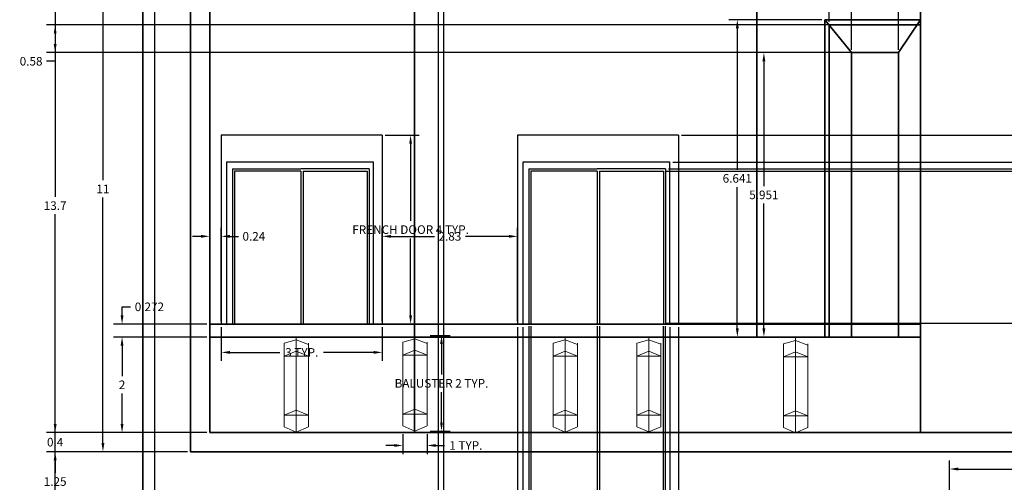
# Model space of a CAD drawing. Units: millimetres. Extents: x 2473 to 2512.3, y 2191.3 to 2230.4.
# Tile 3 of 8: x 2473 to 2493.7, y 2206.4 to 2216.1. Entities that reach past the tile are written whole.
import ezdxf

# ---------------------------------------------------------------- set-up
doc = ezdxf.new("R2010")
doc.units = ezdxf.units.MM
for name, color, linetype, lineweight in [('A-ANNO-DIMS', 2, 'Continuous', 18), ('A-ELEV', 7, 'Continuous', 35), ('A-FLOR-HRAL', 8, 'Continuous', 18), ('A-GLAZ', 3, 'Continuous', 25)]:
    doc.layers.add(name, color=color, linetype=linetype, lineweight=lineweight)
doc.styles.get("Standard").update_dxf_attribs({"font": 'arial.ttf'})
doc.dimstyles.get("Standard").update_dxf_attribs({"dimtxt": 0.18, "dimasz": 0.18, "dimexe": 0.18, "dimexo": 0.0625, "dimgap": 0.09, "dimtad": 0, "dimtih": 1, "dimtoh": 1, "dimdec": 4, "dimzin": 0, "dimdsep": 46, "dimtxsty": 'Standard', "dimcen": 0.09, "dimadec": 0, "dimazin": 0, "dimtfac": 1, "dimtdec": 4, "dimtofl": 0, "dimtmove": 0, "dimatfit": 3, "dimfxl": 1, "dimtolj": 1, "dimtzin": 0, "dimarcsym": 0})

# ---------------------------------------------------------------- blocks, each defined once
blk = doc.blocks.new('BALUSTER')
for p, q in [((0, 1.86), (0.25, 1.93)), ((0, 1.86), (0, 0.108)), ((0.25, 2), (0.25, 0)), ((0.25, 1.93), (0.507, 1.835)), ((0.507, 0.108), (0.507, 1.86)), ((0, 1.589), (0.25, 1.693)), ((0.25, 1.693), (0.507, 1.589)), ((0, 1.589), (0.25, 1.589)), ((0.25, 1.589), (0.507, 1.589)), ((0, 0.354), (0.25, 0.459)), ((0.25, 0.459), (0.507, 0.354)), ((0, 0.354), (0.25, 0.354)), ((0.25, 0.354), (0.507, 0.354)), ((0.25, 0), (0, 0.108)), ((0.25, 0), (0.507, 0.108))]:
    blk.add_line(p, q)
blk = doc.blocks.new('WIN-FRENCH-DOOR')
for p, q in [((0, 3.953), (0, 0)), ((3.371, 3.953), (0, 3.953)), ((3.371, 3.953), (3.371, 0)), ((3.186, 3.385), (0.113, 3.385)), ((0.113, 3.385), (0.113, 0)), ((3.186, 0), (3.186, 3.385)), ((0.234, 3.25), (0.234, 0.02)), ((0.234, 3.25), (1.664, 3.25)), ((1.664, 3.2), (0.275, 3.2)), ((0.275, 3.2), (0.275, 0.02)), ((3.094, 3.25), (1.664, 3.25)), ((1.664, 3.2), (1.664, 0.02)), ((1.664, 3.2), (1.664, 0.02)), ((1.718, 3.2), (3.052, 3.2)), ((1.718, 3.2), (1.718, 0.016)), ((3.052, 3.2), (3.052, 0.02)), ((3.094, 3.25), (3.094, 0.02))]:
    blk.add_line(p, q)
blk = doc.blocks.new('*D3')
at = {"layer": 'A-ANNO-DIMS', "color": 0, "lineweight": -2, "transparency": 16777216}
for p, q in [((2481.638, 2209.486), (2482.056, 2209.486)), ((2481.876, 2209.306), (2481.876, 2208.669)), ((2481.876, 2207.666), (2481.876, 2208.303)), ((2481.638, 2207.486), (2482.056, 2207.486))]:
    blk.add_line(p, q, dxfattribs=at)
at = {"layer": 'A-ANNO-DIMS', "color": 0, "transparency": 16777216}
for points in [[(2481.846, 2209.306), (2481.906, 2209.306), (2481.876, 2209.486)], [(2481.846, 2207.666), (2481.906, 2207.666), (2481.876, 2207.486)]]:
    blk.add_solid(points, dxfattribs=at)
at = {"layer": 'Defpoints', "color": 0, "transparency": 16777216}
for p in [(2481.576, 2209.486), (2481.876, 2209.486), (2481.576, 2207.486)]:
    blk.add_point(p, dxfattribs=at)
at = {"layer": 'A-ANNO-DIMS', "color": 0, "transparency": 16777216, "insert": (2481.876, 2208.486), "char_height": 0.18, "attachment_point": 5}
blk.add_mtext('\\A1;BALUSTER 2 TYP.', dxfattribs=at)
blk = doc.blocks.new('*D4')
at = {"layer": 'A-ANNO-DIMS', "color": 0, "lineweight": -2, "transparency": 16777216}
for p, q in [((2481.069, 2207.423), (2481.069, 2207.006)), ((2481.576, 2207.423), (2481.576, 2207.006)), ((2480.889, 2207.186), (2480.709, 2207.186)), ((2481.756, 2207.186), (2481.936, 2207.186))]:
    blk.add_line(p, q, dxfattribs=at)
at = {"layer": 'A-ANNO-DIMS', "color": 0, "transparency": 16777216}
for points in [[(2480.889, 2207.216), (2480.889, 2207.156), (2481.069, 2207.186)], [(2481.756, 2207.216), (2481.756, 2207.156), (2481.576, 2207.186)]]:
    blk.add_solid(points, dxfattribs=at)
at = {"layer": 'Defpoints', "color": 0, "transparency": 16777216}
for p in [(2481.069, 2207.486), (2481.576, 2207.486), (2481.576, 2207.186)]:
    blk.add_point(p, dxfattribs=at)
at = {"layer": 'A-ANNO-DIMS', "color": 0, "transparency": 16777216, "insert": (2482.386, 2207.186), "char_height": 0.18, "attachment_point": 5}
blk.add_mtext('\\A1;1 TYP.', dxfattribs=at)
blk = doc.blocks.new('*D5')
at = {"layer": 'A-ANNO-DIMS', "color": 0, "lineweight": -2, "transparency": 16777216}
for p, q in [((2480.698, 2213.68), (2481.409, 2213.68)), ((2481.229, 2213.5), (2481.229, 2211.886)), ((2481.229, 2209.907), (2481.229, 2211.52)), ((2480.698, 2209.727), (2481.409, 2209.727))]:
    blk.add_line(p, q, dxfattribs=at)
at = {"layer": 'A-ANNO-DIMS', "color": 0, "transparency": 16777216}
for points in [[(2481.199, 2213.5), (2481.259, 2213.5), (2481.229, 2213.68)], [(2481.199, 2209.907), (2481.259, 2209.907), (2481.229, 2209.727)]]:
    blk.add_solid(points, dxfattribs=at)
at = {"layer": 'Defpoints', "color": 0, "transparency": 16777216}
for p in [(2480.636, 2213.68), (2481.229, 2213.68), (2480.636, 2209.727)]:
    blk.add_point(p, dxfattribs=at)
at = {"layer": 'A-ANNO-DIMS', "color": 0, "transparency": 16777216, "insert": (2481.229, 2211.703), "char_height": 0.18, "attachment_point": 5}
blk.add_mtext('\\A1;FRENCH DOOR 4 TYP.', dxfattribs=at)
blk = doc.blocks.new('*D6')
at = {"layer": 'A-ANNO-DIMS', "color": 0, "lineweight": -2, "transparency": 16777216}
for p, q in [((2477.265, 2209.664), (2477.265, 2208.954)), ((2480.636, 2209.664), (2480.636, 2208.954)), ((2477.445, 2209.134), (2478.492, 2209.134)), ((2480.456, 2209.134), (2479.408, 2209.134))]:
    blk.add_line(p, q, dxfattribs=at)
at = {"layer": 'A-ANNO-DIMS', "color": 0, "transparency": 16777216}
for points in [[(2477.445, 2209.164), (2477.445, 2209.104), (2477.265, 2209.134)], [(2480.456, 2209.164), (2480.456, 2209.104), (2480.636, 2209.134)]]:
    blk.add_solid(points, dxfattribs=at)
at = {"layer": 'Defpoints', "color": 0, "transparency": 16777216}
for p in [(2477.265, 2209.727), (2480.636, 2209.727), (2480.636, 2209.134)]:
    blk.add_point(p, dxfattribs=at)
at = {"layer": 'A-ANNO-DIMS', "color": 0, "transparency": 16777216, "insert": (2478.95, 2209.134), "char_height": 0.18, "attachment_point": 5}
blk.add_mtext('\\A1;3 TYP.', dxfattribs=at)
blk = doc.blocks.new('*D12')
at = {"layer": 'A-ANNO-DIMS', "color": 0, "lineweight": -2, "transparency": 16777216}
for p, q in [((2475.56, 2219.055), (2473.608, 2219.055)), ((2473.788, 2218.875), (2473.788, 2212.387)), ((2473.788, 2205.535), (2473.788, 2212.023)), ((2475.56, 2205.355), (2473.608, 2205.355))]:
    blk.add_line(p, q, dxfattribs=at)
at = {"layer": 'A-ANNO-DIMS', "color": 0, "transparency": 16777216}
for points in [[(2473.758, 2218.875), (2473.818, 2218.875), (2473.788, 2219.055)], [(2473.758, 2205.535), (2473.818, 2205.535), (2473.788, 2205.355)]]:
    blk.add_solid(points, dxfattribs=at)
at = {"layer": 'Defpoints', "color": 0, "transparency": 16777216}
for p in [(2473.788, 2219.055), (2475.623, 2219.055), (2475.623, 2205.355)]:
    blk.add_point(p, dxfattribs=at)
at = {"layer": 'A-ANNO-DIMS', "color": 0, "transparency": 16777216, "insert": (2473.788, 2212.205), "char_height": 0.18, "attachment_point": 5}
blk.add_mtext('\\A1;13.7', dxfattribs=at)
blk = doc.blocks.new('*D19')
at = {"layer": 'A-ANNO-DIMS', "color": 0, "lineweight": -2, "transparency": 16777216}
for p, q in [((2476.56, 2218.055), (2474.608, 2218.055)), ((2474.788, 2217.875), (2474.788, 2212.735)), ((2474.788, 2207.235), (2474.788, 2212.375)), ((2476.56, 2207.055), (2474.608, 2207.055))]:
    blk.add_line(p, q, dxfattribs=at)
at = {"layer": 'A-ANNO-DIMS', "color": 0, "transparency": 16777216}
for points in [[(2474.758, 2217.875), (2474.818, 2217.875), (2474.788, 2218.055)], [(2474.758, 2207.235), (2474.818, 2207.235), (2474.788, 2207.055)]]:
    blk.add_solid(points, dxfattribs=at)
at = {"layer": 'Defpoints', "color": 0, "transparency": 16777216}
for p in [(2474.788, 2218.055), (2476.623, 2218.055), (2476.623, 2207.055)]:
    blk.add_point(p, dxfattribs=at)
at = {"layer": 'A-ANNO-DIMS', "color": 0, "transparency": 16777216, "insert": (2474.788, 2212.555), "char_height": 0.18, "attachment_point": 5}
blk.add_mtext('\\A1;11', dxfattribs=at)
blk = doc.blocks.new('*D38')
at = {"layer": 'A-ANNO-DIMS', "color": 0, "lineweight": -2, "transparency": 16777216}
for p, q in [((2476.56, 2207.055), (2473.608, 2207.055)), ((2473.788, 2206.875), (2473.788, 2206.613)), ((2473.788, 2205.988), (2473.788, 2206.249)), ((2475.56, 2205.808), (2473.608, 2205.808))]:
    blk.add_line(p, q, dxfattribs=at)
at = {"layer": 'A-ANNO-DIMS', "color": 0, "transparency": 16777216}
for points in [[(2473.758, 2206.875), (2473.818, 2206.875), (2473.788, 2207.055)], [(2473.758, 2205.988), (2473.818, 2205.988), (2473.788, 2205.808)]]:
    blk.add_solid(points, dxfattribs=at)
at = {"layer": 'Defpoints', "color": 0, "transparency": 16777216}
for p in [(2473.788, 2207.055), (2476.623, 2207.055), (2475.623, 2205.808)]:
    blk.add_point(p, dxfattribs=at)
at = {"layer": 'A-ANNO-DIMS', "color": 0, "transparency": 16777216, "insert": (2473.788, 2206.431), "char_height": 0.18, "attachment_point": 5}
blk.add_mtext('\\A1;1.25', dxfattribs=at)
blk = doc.blocks.new('*D44')
at = {"layer": 'A-ANNO-DIMS', "color": 0, "lineweight": -2, "transparency": 16777216}
for p, q in [((2492.513, 2204.92), (2492.513, 2206.873)), ((2499.711, 2204.92), (2499.711, 2206.873)), ((2492.693, 2206.693), (2495.719, 2206.693)), ((2499.531, 2206.693), (2496.505, 2206.693))]:
    blk.add_line(p, q, dxfattribs=at)
at = {"layer": 'A-ANNO-DIMS', "color": 0, "transparency": 16777216}
for points in [[(2492.693, 2206.723), (2492.693, 2206.663), (2492.513, 2206.693)], [(2499.531, 2206.723), (2499.531, 2206.663), (2499.711, 2206.693)]]:
    blk.add_solid(points, dxfattribs=at)
at = {"layer": 'Defpoints', "color": 0, "transparency": 16777216}
for p in [(2499.711, 2206.693), (2492.513, 2204.858), (2499.711, 2204.858)]:
    blk.add_point(p, dxfattribs=at)
at = {"layer": 'A-ANNO-DIMS', "color": 0, "transparency": 16777216, "insert": (2496.112, 2206.693), "char_height": 0.18, "attachment_point": 5}
blk.add_mtext('\\A1;7.197', dxfattribs=at)
blk = doc.blocks.new('*D45')
at = {"layer": 'A-ANNO-DIMS', "color": 0, "lineweight": -2, "transparency": 16777216}
for p, q in [((2473.787904, 2207.634888), (2473.787904, 2207.814888)), ((2476.960404, 2207.454888), (2473.607904, 2207.454888)), ((2476.560404, 2207.054888), (2473.607904, 2207.054888)), ((2473.787904, 2206.874888), (2473.787904, 2206.694888))]:
    blk.add_line(p, q, dxfattribs=at)
at = {"layer": 'A-ANNO-DIMS', "color": 0, "transparency": 16777216}
for points in [[(2473.757904, 2207.634888), (2473.817904, 2207.634888), (2473.787904, 2207.454888)], [(2473.757904, 2206.874888), (2473.817904, 2206.874888), (2473.787904, 2207.054888)]]:
    blk.add_solid(points, dxfattribs=at)
at = {"layer": 'Defpoints', "color": 0, "transparency": 16777216}
for p in [(2473.787904, 2207.454888), (2477.022904, 2207.454888), (2476.622904, 2207.054888)]:
    blk.add_point(p, dxfattribs=at)
at = {"layer": 'A-ANNO-DIMS', "color": 0, "transparency": 16777216, "insert": (2473.787904, 2207.254888), "char_height": 0.18, "attachment_point": 5}
blk.add_mtext('\\A1;0.4', dxfattribs=at)
blk = doc.blocks.new('*D52')
at = {"layer": 'A-ANNO-DIMS', "color": 0, "lineweight": -2, "transparency": 16777216}
for p, q in [((2477.023, 2209.789), (2477.023, 2211.742)), ((2477.265, 2209.789), (2477.265, 2211.742)), ((2476.843, 2211.562), (2476.663, 2211.562)), ((2477.445, 2211.562), (2477.625, 2211.562))]:
    blk.add_line(p, q, dxfattribs=at)
at = {"layer": 'A-ANNO-DIMS', "color": 0, "transparency": 16777216}
for points in [[(2476.843, 2211.592), (2476.843, 2211.532), (2477.023, 2211.562)], [(2477.445, 2211.592), (2477.445, 2211.532), (2477.265, 2211.562)]]:
    blk.add_solid(points, dxfattribs=at)
at = {"layer": 'Defpoints', "color": 0, "transparency": 16777216}
for p in [(2477.265, 2211.562), (2477.023, 2209.727), (2477.265, 2209.727)]:
    blk.add_point(p, dxfattribs=at)
at = {"layer": 'A-ANNO-DIMS', "color": 0, "transparency": 16777216, "insert": (2477.948, 2211.562), "char_height": 0.18, "attachment_point": 5}
blk.add_mtext('\\A1;0.24', dxfattribs=at)
blk = doc.blocks.new('*D53')
at = {"layer": 'A-ANNO-DIMS', "color": 0, "lineweight": -2, "transparency": 16777216}
for p, q in [((2480.636, 2209.789), (2480.636, 2211.742)), ((2483.468, 2209.789), (2483.468, 2211.742)), ((2480.816, 2211.562), (2481.727, 2211.562)), ((2483.288, 2211.562), (2482.377, 2211.562))]:
    blk.add_line(p, q, dxfattribs=at)
at = {"layer": 'A-ANNO-DIMS', "color": 0, "transparency": 16777216}
for points in [[(2480.816, 2211.592), (2480.816, 2211.532), (2480.636, 2211.562)], [(2483.288, 2211.592), (2483.288, 2211.532), (2483.468, 2211.562)]]:
    blk.add_solid(points, dxfattribs=at)
at = {"layer": 'Defpoints', "color": 0, "transparency": 16777216}
for p in [(2483.468, 2211.562), (2480.636, 2209.727), (2483.468, 2209.727)]:
    blk.add_point(p, dxfattribs=at)
at = {"layer": 'A-ANNO-DIMS', "color": 0, "transparency": 16777216, "insert": (2482.052, 2211.562), "char_height": 0.18, "attachment_point": 5}
blk.add_mtext('\\A1;2.83', dxfattribs=at)
blk = doc.blocks.new('*D54')
at = {"layer": 'A-ANNO-DIMS', "color": 0, "lineweight": -2, "transparency": 16777216}
for p, q in [((2476.96, 2209.455), (2475.008, 2209.455)), ((2475.188, 2209.275), (2475.188, 2208.635)), ((2475.188, 2207.635), (2475.188, 2208.275)), ((2476.96, 2207.455), (2475.008, 2207.455))]:
    blk.add_line(p, q, dxfattribs=at)
at = {"layer": 'A-ANNO-DIMS', "color": 0, "transparency": 16777216}
for points in [[(2475.158, 2209.275), (2475.218, 2209.275), (2475.188, 2209.455)], [(2475.158, 2207.635), (2475.218, 2207.635), (2475.188, 2207.455)]]:
    blk.add_solid(points, dxfattribs=at)
at = {"layer": 'Defpoints', "color": 0, "transparency": 16777216}
for p in [(2475.188, 2209.455), (2477.023, 2209.455), (2477.023, 2207.455)]:
    blk.add_point(p, dxfattribs=at)
at = {"layer": 'A-ANNO-DIMS', "color": 0, "transparency": 16777216, "insert": (2475.188, 2208.455), "char_height": 0.18, "attachment_point": 5}
blk.add_mtext('\\A1;2', dxfattribs=at)
blk = doc.blocks.new('*D55')
at = {"layer": 'A-ANNO-DIMS', "color": 0, "lineweight": -2, "transparency": 16777216}
for p, q in [((2475.188, 2209.907), (2475.188, 2210.087)), ((2475.188, 2210.087), (2475.368, 2210.087)), ((2476.96, 2209.727), (2475.008, 2209.727)), ((2476.96, 2209.455), (2475.008, 2209.455)), ((2475.188, 2209.275), (2475.188, 2209.095))]:
    blk.add_line(p, q, dxfattribs=at)
at = {"layer": 'A-ANNO-DIMS', "color": 0, "transparency": 16777216}
for points in [[(2475.158, 2209.907), (2475.218, 2209.907), (2475.188, 2209.727)], [(2475.158, 2209.275), (2475.218, 2209.275), (2475.188, 2209.455)]]:
    blk.add_solid(points, dxfattribs=at)
at = {"layer": 'Defpoints', "color": 0, "transparency": 16777216}
for p in [(2475.188, 2209.727), (2477.023, 2209.727), (2477.023, 2209.455)]:
    blk.add_point(p, dxfattribs=at)
at = {"layer": 'A-ANNO-DIMS', "color": 0, "transparency": 16777216, "insert": (2475.761, 2210.087), "char_height": 0.18, "attachment_point": 5}
blk.add_mtext('\\A1;0.272', dxfattribs=at)
blk = doc.blocks.new('*D58')
at = {"layer": 'A-ANNO-DIMS', "color": 0, "lineweight": -2, "transparency": 16777216}
for p, q in [((2490.46, 2215.468), (2490.46, 2217.421)), ((2491.441, 2215.468), (2491.441, 2217.421)), ((2490.28, 2217.241), (2490.1, 2217.241)), ((2491.621, 2217.241), (2491.801, 2217.241))]:
    blk.add_line(p, q, dxfattribs=at)
at = {"layer": 'A-ANNO-DIMS', "color": 0, "transparency": 16777216}
for points in [[(2490.28, 2217.271), (2490.28, 2217.211), (2490.46, 2217.241)], [(2491.621, 2217.271), (2491.621, 2217.211), (2491.441, 2217.241)]]:
    blk.add_solid(points, dxfattribs=at)
at = {"layer": 'Defpoints', "color": 0, "transparency": 16777216}
for p in [(2491.441, 2217.241), (2490.46, 2215.406), (2491.441, 2215.406)]:
    blk.add_point(p, dxfattribs=at)
at = {"layer": 'A-ANNO-DIMS', "color": 0, "transparency": 16777216, "insert": (2490.95, 2217.241), "char_height": 0.18, "attachment_point": 5}
blk.add_mtext('\\A1;0.981', dxfattribs=at)
blk = doc.blocks.new('*D59')
at = {"layer": 'A-ANNO-DIMS', "color": 0, "lineweight": -2, "transparency": 16777216}
for p, q in [((2489.841, 2216.096), (2487.889, 2216.096)), ((2488.069, 2215.916), (2488.069, 2212.957)), ((2488.069, 2209.635), (2488.069, 2212.593)), ((2489.841, 2209.455), (2487.889, 2209.455))]:
    blk.add_line(p, q, dxfattribs=at)
at = {"layer": 'A-ANNO-DIMS', "color": 0, "transparency": 16777216}
for points in [[(2488.039, 2215.916), (2488.099, 2215.916), (2488.069, 2216.096)], [(2488.039, 2209.635), (2488.099, 2209.635), (2488.069, 2209.455)]]:
    blk.add_solid(points, dxfattribs=at)
at = {"layer": 'Defpoints', "color": 0, "transparency": 16777216}
for p in [(2488.069, 2216.096), (2489.904, 2216.096), (2489.904, 2209.455)]:
    blk.add_point(p, dxfattribs=at)
at = {"layer": 'A-ANNO-DIMS', "color": 0, "transparency": 16777216, "insert": (2488.069, 2212.775), "char_height": 0.18, "attachment_point": 5}
blk.add_mtext('\\A1;6.641', dxfattribs=at)
blk = doc.blocks.new('*D60')
at = {"layer": 'A-ANNO-DIMS', "color": 0, "lineweight": -2, "transparency": 16777216}
for p, q in [((2490.397, 2215.406), (2488.445, 2215.406)), ((2488.625, 2215.226), (2488.625, 2212.612)), ((2488.625, 2209.635), (2488.625, 2212.249)), ((2490.397, 2209.455), (2488.445, 2209.455))]:
    blk.add_line(p, q, dxfattribs=at)
at = {"layer": 'A-ANNO-DIMS', "color": 0, "transparency": 16777216}
for points in [[(2488.595, 2215.226), (2488.655, 2215.226), (2488.625, 2215.406)], [(2488.595, 2209.635), (2488.655, 2209.635), (2488.625, 2209.455)]]:
    blk.add_solid(points, dxfattribs=at)
at = {"layer": 'Defpoints', "color": 0, "transparency": 16777216}
for p in [(2488.625, 2215.406), (2490.46, 2215.406), (2490.46, 2209.455)]:
    blk.add_point(p, dxfattribs=at)
at = {"layer": 'A-ANNO-DIMS', "color": 0, "transparency": 16777216, "insert": (2488.625, 2212.43), "char_height": 0.18, "attachment_point": 5}
blk.add_mtext('\\A1;5.951', dxfattribs=at)
blk = doc.blocks.new('*D99')
at = {"layer": 'A-ANNO-DIMS', "color": 0, "lineweight": -2, "transparency": 16777216}
for p, q in [((2491.841, 2215.987), (2473.608, 2215.987)), ((2473.788, 2215.807), (2473.788, 2215.586)), ((2491.378, 2215.406), (2473.608, 2215.406)), ((2473.788, 2215.406), (2473.788, 2215.226)), ((2473.788, 2215.226), (2473.608, 2215.226))]:
    blk.add_line(p, q, dxfattribs=at)
at = {"layer": 'A-ANNO-DIMS', "color": 0, "transparency": 16777216}
for points in [[(2473.758, 2215.807), (2473.818, 2215.807), (2473.788, 2215.987)], [(2473.758, 2215.586), (2473.818, 2215.586), (2473.788, 2215.406)]]:
    blk.add_solid(points, dxfattribs=at)
at = {"layer": 'Defpoints', "color": 0, "transparency": 16777216}
for p in [(2491.904, 2215.987), (2473.788, 2215.406), (2491.441, 2215.406)]:
    blk.add_point(p, dxfattribs=at)
at = {"layer": 'A-ANNO-DIMS', "color": 0, "transparency": 16777216, "insert": (2473.284, 2215.226), "char_height": 0.18, "attachment_point": 5}
blk.add_mtext('\\A1;0.58', dxfattribs=at)
blk = doc.blocks.new('*D100')
at = {"layer": 'A-ANNO-DIMS', "color": 0, "lineweight": -2, "transparency": 16777216}
for p, q in [((2489.991, 2216.05), (2489.991, 2230.37)), ((2490.46, 2215.468), (2490.46, 2230.37)), ((2489.811, 2230.19), (2489.631, 2230.19)), ((2490.64, 2230.19), (2490.82, 2230.19))]:
    blk.add_line(p, q, dxfattribs=at)
at = {"layer": 'A-ANNO-DIMS', "color": 0, "transparency": 16777216}
for points in [[(2489.811, 2230.22), (2489.811, 2230.16), (2489.991, 2230.19)], [(2490.64, 2230.22), (2490.64, 2230.16), (2490.46, 2230.19)]]:
    blk.add_solid(points, dxfattribs=at)
at = {"layer": 'Defpoints', "color": 0, "transparency": 16777216}
for p in [(2490.46, 2230.19), (2489.991, 2215.987), (2490.46, 2215.406)]:
    blk.add_point(p, dxfattribs=at)
at = {"layer": 'A-ANNO-DIMS', "color": 0, "transparency": 16777216, "insert": (2491.143, 2230.19), "char_height": 0.18, "attachment_point": 5}
blk.add_mtext('\\A1;0.47', dxfattribs=at)
blk = doc.blocks.new('*D101')
at = {"layer": 'A-ANNO-DIMS', "color": 0, "lineweight": -2, "transparency": 16777216}
for p, q in [((2491.441, 2215.468), (2491.441, 2230.37)), ((2491.904, 2216.05), (2491.904, 2230.37)), ((2491.261, 2230.19), (2491.081, 2230.19)), ((2492.084, 2230.19), (2492.264, 2230.19))]:
    blk.add_line(p, q, dxfattribs=at)
at = {"layer": 'A-ANNO-DIMS', "color": 0, "transparency": 16777216}
for points in [[(2491.261, 2230.22), (2491.261, 2230.16), (2491.441, 2230.19)], [(2492.084, 2230.22), (2492.084, 2230.16), (2491.904, 2230.19)]]:
    blk.add_solid(points, dxfattribs=at)
at = {"layer": 'Defpoints', "color": 0, "transparency": 16777216}
for p in [(2491.904, 2230.19), (2491.904, 2215.987), (2491.441, 2215.406)]:
    blk.add_point(p, dxfattribs=at)
at = {"layer": 'A-ANNO-DIMS', "color": 0, "transparency": 16777216, "insert": (2492.587, 2230.19), "char_height": 0.18, "attachment_point": 5}
blk.add_mtext('\\A1;0.46', dxfattribs=at)
blk = doc.blocks.new('*D102')
at = {"layer": 'A-ANNO-DIMS', "color": 0, "lineweight": -2, "transparency": 16777216}
for p, q in [((2483.468, 2209.664), (2483.468, 2191.34)), ((2483.581, 2209.664), (2483.581, 2191.34)), ((2483.288, 2191.52), (2483.108, 2191.52)), ((2483.761, 2191.52), (2483.941, 2191.52))]:
    blk.add_line(p, q, dxfattribs=at)
at = {"layer": 'A-ANNO-DIMS', "color": 0, "transparency": 16777216}
for points in [[(2483.288, 2191.55), (2483.288, 2191.49), (2483.468, 2191.52)], [(2483.761, 2191.55), (2483.761, 2191.49), (2483.581, 2191.52)]]:
    blk.add_solid(points, dxfattribs=at)
at = {"layer": 'Defpoints', "color": 0, "transparency": 16777216}
for p in [(2483.468, 2209.727), (2483.581, 2209.727), (2483.581, 2191.52)]:
    blk.add_point(p, dxfattribs=at)
at = {"layer": 'A-ANNO-DIMS', "color": 0, "transparency": 16777216, "insert": (2484.248, 2191.52), "char_height": 0.18, "attachment_point": 5}
blk.add_mtext('\\A1;0.11', dxfattribs=at)
blk = doc.blocks.new('*D103')
at = {"layer": 'A-ANNO-DIMS', "color": 0, "lineweight": -2, "transparency": 16777216}
for p, q in [((2483.581, 2209.664), (2483.581, 2191.34)), ((2483.702, 2209.684), (2483.702, 2191.34)), ((2483.401, 2191.52), (2483.221, 2191.52)), ((2483.882, 2191.52), (2484.062, 2191.52))]:
    blk.add_line(p, q, dxfattribs=at)
at = {"layer": 'A-ANNO-DIMS', "color": 0, "transparency": 16777216}
for points in [[(2483.401, 2191.55), (2483.401, 2191.49), (2483.581, 2191.52)], [(2483.882, 2191.55), (2483.882, 2191.49), (2483.702, 2191.52)]]:
    blk.add_solid(points, dxfattribs=at)
at = {"layer": 'Defpoints', "color": 0, "transparency": 16777216}
for p in [(2483.702, 2209.747), (2483.581, 2209.727), (2483.702, 2191.52)]:
    blk.add_point(p, dxfattribs=at)
at = {"layer": 'A-ANNO-DIMS', "color": 0, "transparency": 16777216, "insert": (2484.439, 2191.52), "char_height": 0.18, "attachment_point": 5}
blk.add_mtext('\\A1;0.121', dxfattribs=at)
blk = doc.blocks.new('*D104')
at = {"layer": 'A-ANNO-DIMS', "color": 0, "lineweight": -2, "transparency": 16777216}
for p, q in [((2483.702, 2209.684), (2483.702, 2191.34)), ((2483.744, 2209.684), (2483.744, 2191.34)), ((2483.522, 2191.52), (2483.342, 2191.52)), ((2483.924, 2191.52), (2484.104, 2191.52))]:
    blk.add_line(p, q, dxfattribs=at)
at = {"layer": 'A-ANNO-DIMS', "color": 0, "transparency": 16777216}
for points in [[(2483.522, 2191.55), (2483.522, 2191.49), (2483.702, 2191.52)], [(2483.924, 2191.55), (2483.924, 2191.49), (2483.744, 2191.52)]]:
    blk.add_solid(points, dxfattribs=at)
at = {"layer": 'Defpoints', "color": 0, "transparency": 16777216}
for p in [(2483.702, 2209.747), (2483.744, 2209.747), (2483.744, 2191.52)]:
    blk.add_point(p, dxfattribs=at)
at = {"layer": 'A-ANNO-DIMS', "color": 0, "transparency": 16777216, "insert": (2484.497, 2191.52), "char_height": 0.18, "attachment_point": 5}
blk.add_mtext('\\A1;0.042', dxfattribs=at)
blk = doc.blocks.new('*D105')
at = {"layer": 'A-ANNO-DIMS', "color": 0, "lineweight": -2, "transparency": 16777216}
for p, q in [((2483.744, 2209.684), (2483.744, 2191.34)), ((2485.132, 2209.684), (2485.132, 2191.34)), ((2483.924, 2191.52), (2484.123, 2191.52)), ((2484.952, 2191.52), (2484.754, 2191.52))]:
    blk.add_line(p, q, dxfattribs=at)
at = {"layer": 'A-ANNO-DIMS', "color": 0, "transparency": 16777216}
for points in [[(2483.924, 2191.55), (2483.924, 2191.49), (2483.744, 2191.52)], [(2484.952, 2191.55), (2484.952, 2191.49), (2485.132, 2191.52)]]:
    blk.add_solid(points, dxfattribs=at)
at = {"layer": 'Defpoints', "color": 0, "transparency": 16777216}
for p in [(2483.744, 2209.747), (2485.132, 2209.747), (2485.132, 2191.52)]:
    blk.add_point(p, dxfattribs=at)
at = {"layer": 'A-ANNO-DIMS', "color": 0, "transparency": 16777216, "insert": (2484.438, 2191.52), "char_height": 0.18, "attachment_point": 5}
blk.add_mtext('\\A1;1.39', dxfattribs=at)
blk = doc.blocks.new('*D106')
at = {"layer": 'A-ANNO-DIMS', "color": 0, "lineweight": -2, "transparency": 16777216}
for p, q in [((2485.132, 2209.684), (2485.132, 2191.34)), ((2485.187, 2209.68), (2485.187, 2191.34)), ((2484.952, 2191.52), (2484.772, 2191.52)), ((2485.367, 2191.52), (2485.547, 2191.52))]:
    blk.add_line(p, q, dxfattribs=at)
at = {"layer": 'A-ANNO-DIMS', "color": 0, "transparency": 16777216}
for points in [[(2484.952, 2191.55), (2484.952, 2191.49), (2485.132, 2191.52)], [(2485.367, 2191.55), (2485.367, 2191.49), (2485.187, 2191.52)]]:
    blk.add_solid(points, dxfattribs=at)
at = {"layer": 'Defpoints', "color": 0, "transparency": 16777216}
for p in [(2485.132, 2209.747), (2485.187, 2209.743), (2485.187, 2191.52)]:
    blk.add_point(p, dxfattribs=at)
at = {"layer": 'A-ANNO-DIMS', "color": 0, "transparency": 16777216, "insert": (2485.871, 2191.52), "char_height": 0.18, "attachment_point": 5}
blk.add_mtext('\\A1;0.05', dxfattribs=at)
blk = doc.blocks.new('*D107')
at = {"layer": 'A-ANNO-DIMS', "color": 0, "lineweight": -2, "transparency": 16777216}
for p, q in [((2485.187, 2209.68), (2485.187, 2191.34)), ((2486.52, 2209.684), (2486.52, 2191.34)), ((2485.367, 2191.52), (2485.469, 2191.52)), ((2486.34, 2191.52), (2486.238, 2191.52))]:
    blk.add_line(p, q, dxfattribs=at)
at = {"layer": 'A-ANNO-DIMS', "color": 0, "transparency": 16777216}
for points in [[(2485.367, 2191.55), (2485.367, 2191.49), (2485.187, 2191.52)], [(2486.34, 2191.55), (2486.34, 2191.49), (2486.52, 2191.52)]]:
    blk.add_solid(points, dxfattribs=at)
at = {"layer": 'Defpoints', "color": 0, "transparency": 16777216}
for p in [(2485.187, 2209.743), (2486.52, 2209.747), (2486.52, 2191.52)]:
    blk.add_point(p, dxfattribs=at)
at = {"layer": 'A-ANNO-DIMS', "color": 0, "transparency": 16777216, "insert": (2485.854, 2191.52), "char_height": 0.18, "attachment_point": 5}
blk.add_mtext('\\A1;1.334', dxfattribs=at)
blk = doc.blocks.new('*D108')
at = {"layer": 'A-ANNO-DIMS', "color": 0, "lineweight": -2, "transparency": 16777216}
for p, q in [((2486.52, 2209.684), (2486.52, 2191.34)), ((2486.562, 2209.684), (2486.562, 2191.34)), ((2486.34, 2191.52), (2486.16, 2191.52)), ((2486.742, 2191.52), (2486.922, 2191.52))]:
    blk.add_line(p, q, dxfattribs=at)
at = {"layer": 'A-ANNO-DIMS', "color": 0, "transparency": 16777216}
for points in [[(2486.34, 2191.55), (2486.34, 2191.49), (2486.52, 2191.52)], [(2486.742, 2191.55), (2486.742, 2191.49), (2486.562, 2191.52)]]:
    blk.add_solid(points, dxfattribs=at)
at = {"layer": 'Defpoints', "color": 0, "transparency": 16777216}
for p in [(2486.52, 2209.747), (2486.562, 2209.747), (2486.562, 2191.52)]:
    blk.add_point(p, dxfattribs=at)
at = {"layer": 'A-ANNO-DIMS', "color": 0, "transparency": 16777216, "insert": (2487.315, 2191.52), "char_height": 0.18, "attachment_point": 5}
blk.add_mtext('\\A1;0.042', dxfattribs=at)
blk = doc.blocks.new('*D109')
at = {"layer": 'A-ANNO-DIMS', "color": 0, "lineweight": -2, "transparency": 16777216}
for p, q in [((2486.562, 2209.684), (2486.562, 2191.34)), ((2486.655, 2209.664), (2486.655, 2191.34)), ((2486.382, 2191.52), (2486.202, 2191.52)), ((2486.835, 2191.52), (2487.015, 2191.52))]:
    blk.add_line(p, q, dxfattribs=at)
at = {"layer": 'A-ANNO-DIMS', "color": 0, "transparency": 16777216}
for points in [[(2486.382, 2191.55), (2486.382, 2191.49), (2486.562, 2191.52)], [(2486.835, 2191.55), (2486.835, 2191.49), (2486.655, 2191.52)]]:
    blk.add_solid(points, dxfattribs=at)
at = {"layer": 'Defpoints', "color": 0, "transparency": 16777216}
for p in [(2486.562, 2209.747), (2486.655, 2209.727), (2486.655, 2191.52)]:
    blk.add_point(p, dxfattribs=at)
at = {"layer": 'A-ANNO-DIMS', "color": 0, "transparency": 16777216, "insert": (2487.339, 2191.52), "char_height": 0.18, "attachment_point": 5}
blk.add_mtext('\\A1;0.09', dxfattribs=at)
blk = doc.blocks.new('*D110')
at = {"layer": 'A-ANNO-DIMS', "color": 0, "lineweight": -2, "transparency": 16777216}
for p, q in [((2486.655, 2209.664), (2486.655, 2191.34)), ((2486.84, 2209.664), (2486.84, 2191.34)), ((2486.475, 2191.52), (2486.295, 2191.52)), ((2487.02, 2191.52), (2487.2, 2191.52))]:
    blk.add_line(p, q, dxfattribs=at)
at = {"layer": 'A-ANNO-DIMS', "color": 0, "transparency": 16777216}
for points in [[(2486.475, 2191.55), (2486.475, 2191.49), (2486.655, 2191.52)], [(2487.02, 2191.55), (2487.02, 2191.49), (2486.84, 2191.52)]]:
    blk.add_solid(points, dxfattribs=at)
at = {"layer": 'Defpoints', "color": 0, "transparency": 16777216}
for p in [(2486.655, 2209.727), (2486.84, 2209.727), (2486.84, 2191.52)]:
    blk.add_point(p, dxfattribs=at)
at = {"layer": 'A-ANNO-DIMS', "color": 0, "transparency": 16777216, "insert": (2487.524, 2191.52), "char_height": 0.18, "attachment_point": 5}
blk.add_mtext('\\A1;0.18', dxfattribs=at)
blk = doc.blocks.new('*D111')
at = {"layer": 'A-ANNO-DIMS', "color": 0, "lineweight": -2, "transparency": 16777216}
for p, q in [((2486.902, 2213.68), (2511.728, 2213.68)), ((2511.548, 2213.5), (2511.548, 2213.292)), ((2486.718, 2213.112), (2511.728, 2213.112)), ((2511.548, 2213.112), (2511.548, 2212.932)), ((2511.548, 2212.932), (2511.368, 2212.932))]:
    blk.add_line(p, q, dxfattribs=at)
at = {"layer": 'A-ANNO-DIMS', "color": 0, "transparency": 16777216}
for points in [[(2511.518, 2213.5), (2511.578, 2213.5), (2511.548, 2213.68)], [(2511.518, 2213.292), (2511.578, 2213.292), (2511.548, 2213.112)]]:
    blk.add_solid(points, dxfattribs=at)
at = {"layer": 'Defpoints', "color": 0, "transparency": 16777216}
for p in [(2486.84, 2213.68), (2486.655, 2213.112), (2511.548, 2213.112)]:
    blk.add_point(p, dxfattribs=at)
at = {"layer": 'A-ANNO-DIMS', "color": 0, "transparency": 16777216, "insert": (2511.044, 2212.932), "char_height": 0.18, "attachment_point": 5}
blk.add_mtext('\\A1;0.57', dxfattribs=at)
blk = doc.blocks.new('*D112')
at = {"layer": 'A-ANNO-DIMS', "color": 0, "lineweight": -2, "transparency": 16777216}
for p, q in [((2511.548, 2213.292), (2511.548, 2213.472)), ((2486.718, 2213.112), (2511.728, 2213.112)), ((2486.625, 2212.977), (2511.728, 2212.977)), ((2511.548, 2212.617), (2511.368, 2212.617)), ((2511.548, 2212.797), (2511.548, 2212.617))]:
    blk.add_line(p, q, dxfattribs=at)
at = {"layer": 'A-ANNO-DIMS', "color": 0, "transparency": 16777216}
for points in [[(2511.518, 2213.292), (2511.578, 2213.292), (2511.548, 2213.112)], [(2511.518, 2212.797), (2511.578, 2212.797), (2511.548, 2212.977)]]:
    blk.add_solid(points, dxfattribs=at)
at = {"layer": 'Defpoints', "color": 0, "transparency": 16777216}
for p in [(2486.655, 2213.112), (2486.562, 2212.977), (2511.548, 2212.977)]:
    blk.add_point(p, dxfattribs=at)
at = {"layer": 'A-ANNO-DIMS', "color": 0, "transparency": 16777216, "insert": (2511.044, 2212.617), "char_height": 0.18, "attachment_point": 5}
blk.add_mtext('\\A1;0.13', dxfattribs=at)
blk = doc.blocks.new('*D113')
at = {"layer": 'A-ANNO-DIMS', "color": 0, "lineweight": -2, "transparency": 16777216}
for p, q in [((2511.548, 2213.157), (2511.548, 2213.337)), ((2486.583, 2212.927), (2511.728, 2212.927)), ((2486.625, 2212.977), (2511.728, 2212.977)), ((2511.548, 2212.747), (2511.548, 2212.567)), ((2511.548, 2212.567), (2511.368, 2212.567))]:
    blk.add_line(p, q, dxfattribs=at)
at = {"layer": 'A-ANNO-DIMS', "color": 0, "transparency": 16777216}
for points in [[(2511.518, 2213.157), (2511.578, 2213.157), (2511.548, 2212.977)], [(2511.518, 2212.747), (2511.578, 2212.747), (2511.548, 2212.927)]]:
    blk.add_solid(points, dxfattribs=at)
at = {"layer": 'Defpoints', "color": 0, "transparency": 16777216}
for p in [(2486.52, 2212.927), (2486.562, 2212.977), (2511.548, 2212.927)]:
    blk.add_point(p, dxfattribs=at)
at = {"layer": 'A-ANNO-DIMS', "color": 0, "transparency": 16777216, "insert": (2511.043, 2212.567), "char_height": 0.18, "attachment_point": 5}
blk.add_mtext('\\A1;0.05', dxfattribs=at)
blk = doc.blocks.new('*D114')
at = {"layer": 'A-ANNO-DIMS', "color": 0, "lineweight": -2, "transparency": 16777216}
for p, q in [((2486.583, 2212.927), (2511.728, 2212.927)), ((2511.548, 2212.747), (2511.548, 2211.519)), ((2511.548, 2209.927), (2511.548, 2211.155)), ((2486.583, 2209.747), (2511.728, 2209.747))]:
    blk.add_line(p, q, dxfattribs=at)
at = {"layer": 'A-ANNO-DIMS', "color": 0, "transparency": 16777216}
for points in [[(2511.518, 2212.747), (2511.578, 2212.747), (2511.548, 2212.927)], [(2511.518, 2209.927), (2511.578, 2209.927), (2511.548, 2209.747)]]:
    blk.add_solid(points, dxfattribs=at)
at = {"layer": 'Defpoints', "color": 0, "transparency": 16777216}
for p in [(2486.52, 2212.927), (2486.52, 2209.747), (2511.548, 2209.747)]:
    blk.add_point(p, dxfattribs=at)
at = {"layer": 'A-ANNO-DIMS', "color": 0, "transparency": 16777216, "insert": (2511.548, 2211.337), "char_height": 0.18, "attachment_point": 5}
blk.add_mtext('\\A1;3.18', dxfattribs=at)
blk = doc.blocks.new('*D126')
at = {"layer": 'A-ANNO-DIMS', "color": 0, "lineweight": -2, "transparency": 16777216}
for p, q in [((2475.623, 2222.992), (2475.623, 2191.34)), ((2475.869, 2223.101), (2475.869, 2191.34)), ((2475.443, 2191.52), (2475.263, 2191.52)), ((2476.049, 2191.52), (2476.229, 2191.52))]:
    blk.add_line(p, q, dxfattribs=at)
at = {"layer": 'A-ANNO-DIMS', "color": 0, "transparency": 16777216}
for points in [[(2475.443, 2191.55), (2475.443, 2191.49), (2475.623, 2191.52)], [(2476.049, 2191.55), (2476.049, 2191.49), (2475.869, 2191.52)]]:
    blk.add_solid(points, dxfattribs=at)
at = {"layer": 'Defpoints', "color": 0, "transparency": 16777216}
for p in [(2475.869, 2223.163), (2475.623, 2223.055), (2475.869, 2191.52)]:
    blk.add_point(p, dxfattribs=at)
at = {"layer": 'A-ANNO-DIMS', "color": 0, "transparency": 16777216, "insert": (2476.553, 2191.52), "char_height": 0.18, "attachment_point": 5}
blk.add_mtext('\\A1;0.25', dxfattribs=at)
blk = doc.blocks.new('*D129')
at = {"layer": 'A-ANNO-DIMS', "color": 0, "lineweight": -2, "transparency": 16777216}
for p, q in [((2481.806, 2223.101), (2481.806, 2191.34)), ((2481.915, 2222.992), (2481.915, 2191.34)), ((2481.626, 2191.52), (2481.446, 2191.52)), ((2482.095, 2191.52), (2482.275, 2191.52))]:
    blk.add_line(p, q, dxfattribs=at)
at = {"layer": 'A-ANNO-DIMS', "color": 0, "transparency": 16777216}
for points in [[(2481.626, 2191.55), (2481.626, 2191.49), (2481.806, 2191.52)], [(2482.095, 2191.55), (2482.095, 2191.49), (2481.915, 2191.52)]]:
    blk.add_solid(points, dxfattribs=at)
at = {"layer": 'Defpoints', "color": 0, "transparency": 16777216}
for p in [(2481.806, 2223.163), (2481.915, 2223.055), (2481.915, 2191.52)]:
    blk.add_point(p, dxfattribs=at)
at = {"layer": 'A-ANNO-DIMS', "color": 0, "transparency": 16777216, "insert": (2482.582, 2191.52), "char_height": 0.18, "attachment_point": 5}
blk.add_mtext('\\A1;0.11', dxfattribs=at)

msp = doc.modelspace()

# ---------------------------------------------------------------- linework, layer by layer
at = {"layer": 'A-ELEV'}
for p, q in [((2475.6229, 2193.3549), (2475.6229, 2219.0549)), ((2476.6229, 2218.0549), (2476.6229, 2207.0549)), ((2477.0229, 2217.6549), (2477.0229, 2207.4549)), ((2481.3096, 2209.4549), (2481.3096, 2217.6549)), ((2488.4789, 2209.4549), (2488.4789, 2217.6549)), ((2491.9035, 2217.6549), (2491.9035, 2207.4549)), ((2491.9035, 2216.0958), (2489.9035, 2216.0958)), ((2489.9035, 2216.0958), (2489.9035, 2209.4549)), ((2489.9035, 2216.0958), (2490.4596, 2215.406)), ((2489.9911, 2215.9871), (2491.9035, 2215.9871)), ((2489.9911, 2215.9871), (2489.9911, 2209.4549)), ((2491.4406, 2215.406), (2491.9035, 2216.0958)), ((2490.4596, 2215.406), (2491.4406, 2215.406)), ((2490.4596, 2215.406), (2490.4596, 2209.4549)), ((2491.4406, 2215.406), (2491.4406, 2209.4549)), ((2491.9035, 2209.7269), (2477.0229, 2209.7269)), ((2491.9035, 2209.4549), (2477.0229, 2209.4549)), ((2481.3096, 2209.4549), (2481.3096, 2207.4549)), ((2477.0229, 2207.4549), (2497.9035, 2207.4549)), ((2476.6229, 2207.0549), (2498.2167, 2207.0549))]:
    msp.add_line(p, q, dxfattribs=at)

# ---------------------------------------------------------------- block references
at = {"layer": 'A-FLOR-HRAL'}
for p in [(2478.5842, 2207.4672), (2481.069, 2207.486), (2484.2159, 2207.4672), (2485.9634, 2207.4681), (2489.0376, 2207.4509)]:
    msp.add_blockref('BALUSTER', p, dxfattribs=at)
at = {"layer": 'A-GLAZ'}
for p in [(2477.265, 2209.727), (2483.4687, 2209.727)]:
    msp.add_blockref('WIN-FRENCH-DOOR', p, dxfattribs=at)

# ---------------------------------------------------------------- dimensions: what is measured, and where the dimension line sits
at = {"layer": 'A-ANNO-DIMS'}
for base, p1, p2, override, picture, middle in [((2490.4596, 2230.1899), (2489.9911, 2215.9871), (2490.4596, 2215.406), {"dimdec": 2, "dimlfac": 1, "dimrnd": 0, "dimzin": 0, "dimdsep": 46, "dimlunit": 2}, '*D100', (2491.1434, 2230.1899)), ((2491.9035, 2230.1899), (2491.4406, 2215.406), (2491.9035, 2215.9871), {"dimdec": 2, "dimlfac": 1, "dimrnd": 0, "dimzin": 0, "dimdsep": 46, "dimlunit": 2}, '*D101', (2492.5872, 2230.1899)), ((2475.869, 2191.5199), (2475.6229, 2223.0549), (2475.869, 2223.1632), {"dimdec": 2, "dimlfac": 1, "dimrnd": 0, "dimzin": 0, "dimdsep": 46, "dimlunit": 2}, '*D126', (2476.5535, 2191.5199)), ((2481.9154, 2191.5199), (2481.806, 2223.1632), (2481.9154, 2223.0549), {"dimdec": 2, "dimlfac": 1, "dimrnd": 0, "dimzin": 0, "dimdsep": 46, "dimlunit": 2}, '*D129', (2482.5818, 2191.5199)), ((2491.4406, 2217.241), (2490.4596, 2215.406), (2491.4406, 2215.406), {"dimdec": 3, "dimlfac": 1, "dimrnd": 0, "dimzin": 0, "dimdsep": 46, "dimlunit": 2}, '*D58', (2490.9501, 2217.241)), ((2477.2646, 2211.5619), (2477.0229, 2209.7269), (2477.2646, 2209.7269), {"dimdec": 2, "dimlfac": 1, "dimrnd": 0, "dimzin": 0, "dimdsep": 46, "dimlunit": 2}, '*D52', (2477.948, 2211.5619)), ((2483.4683, 2211.5619), (2480.6359, 2209.7269), (2483.4683, 2209.7269), {"dimdec": 2, "dimlfac": 1, "dimrnd": 0, "dimzin": 0, "dimdsep": 46, "dimlunit": 2}, '*D53', (2482.0521, 2211.5619)), ((2483.7022, 2191.5199), (2483.5812, 2209.7269), (2483.7022, 2209.7466), {"dimdec": 3, "dimlfac": 1, "dimrnd": 0, "dimzin": 0, "dimdsep": 46, "dimlunit": 2}, '*D103', (2484.4385, 2191.5199)), ((2483.7441, 2191.5199), (2483.7022, 2209.7466), (2483.7441, 2209.7466), {"dimdec": 3, "dimlfac": 1, "dimrnd": 0, "dimzin": 0, "dimdsep": 46, "dimlunit": 2}, '*D104', (2484.4969, 2191.5199)), ((2485.1323, 2191.5199), (2483.7441, 2209.7466), (2485.1323, 2209.7466), {"dimdec": 2, "dimlfac": 1, "dimrnd": 0, "dimzin": 0, "dimdsep": 46, "dimlunit": 2}, '*D105', (2484.4382, 2191.5199)), ((2485.1866, 2191.5199), (2485.1323, 2209.7466), (2485.1866, 2209.7428), {"dimdec": 2, "dimlfac": 1, "dimrnd": 0, "dimzin": 0, "dimdsep": 46, "dimlunit": 2}, '*D106', (2485.871, 2191.5199)), ((2486.5205, 2191.5199), (2485.1866, 2209.7428), (2486.5205, 2209.7466), {"dimdec": 3, "dimlfac": 1, "dimrnd": 0, "dimzin": 0, "dimdsep": 46, "dimlunit": 2}, '*D107', (2485.8535, 2191.5199)), ((2486.5624, 2191.5199), (2486.5205, 2209.7466), (2486.5624, 2209.7466), {"dimdec": 3, "dimlfac": 1, "dimrnd": 0, "dimzin": 0, "dimdsep": 46, "dimlunit": 2}, '*D108', (2487.3152, 2191.5199)), ((2486.655, 2191.5199), (2486.5624, 2209.7466), (2486.655, 2209.7269), {"dimdec": 2, "dimlfac": 1, "dimrnd": 0, "dimzin": 0, "dimdsep": 46, "dimlunit": 2}, '*D109', (2487.339, 2191.5199)), ((2483.5812, 2191.5199), (2483.4683, 2209.7269), (2483.5812, 2209.7269), {"dimdec": 2, "dimlfac": 1, "dimrnd": 0, "dimzin": 0, "dimdsep": 46, "dimlunit": 2}, '*D102', (2484.2476, 2191.5199)), ((2486.8395, 2191.5199), (2486.655, 2209.7269), (2486.8395, 2209.7269), {"dimdec": 2, "dimlfac": 1, "dimrnd": 0, "dimzin": 0, "dimdsep": 46, "dimlunit": 2}, '*D110', (2487.5235, 2191.5199)), ((2499.7107, 2206.6926), (2492.5133, 2204.8576), (2499.7107, 2204.8576), {"dimdec": 3, "dimlfac": 1, "dimrnd": 0, "dimzin": 0, "dimdsep": 46, "dimlunit": 2}, '*D44', (2496.112, 2206.6926))]:
    dim = msp.add_linear_dim(base=base, p1=p1, p2=p2, dimstyle='Standard', override=override, dxfattribs=at)
    dim.commit()
    dim.dimension.update_dxf_attribs({"geometry": picture, "text_midpoint": middle})
for base, p1, p2, override, picture, middle in [((2473.7879, 2219.0549), (2475.6229, 2205.3549), (2475.6229, 2219.0549), {"dimdec": 1, "dimlfac": 1, "dimrnd": 0, "dimzin": 0, "dimdsep": 46, "dimlunit": 2}, '*D12', (2473.7879, 2212.2049)), ((2474.7879, 2218.0549), (2476.6229, 2207.0549), (2476.6229, 2218.0549), {"dimdec": 0, "dimlfac": 1, "dimrnd": 0, "dimzin": 0, "dimdsep": 46, "dimlunit": 2}, '*D19', (2474.7879, 2212.5549)), ((2473.7879, 2215.406), (2491.9035, 2215.9871), (2491.4406, 2215.406), {"dimdec": 2, "dimlfac": 1, "dimrnd": 0, "dimzin": 0, "dimdsep": 46, "dimlunit": 2}, '*D99', (2473.2839, 2215.226)), ((2488.0685, 2216.0958), (2489.9035, 2209.4549), (2489.9035, 2216.0958), {"dimdec": 3, "dimlfac": 1, "dimrnd": 0, "dimzin": 0, "dimdsep": 46, "dimlunit": 2}, '*D59', (2488.0685, 2212.7753)), ((2488.6246, 2215.406), (2490.4596, 2209.4549), (2490.4596, 2215.406), {"dimdec": 3, "dimlfac": 1, "dimrnd": 0, "dimzin": 0, "dimdsep": 46, "dimlunit": 2}, '*D60', (2488.6246, 2212.4304)), ((2511.5479, 2213.1115), (2486.8395, 2213.6797), (2486.655, 2213.1115), {"dimdec": 2, "dimlfac": 1, "dimrnd": 0, "dimzin": 0, "dimdsep": 46, "dimlunit": 2}, '*D111', (2511.0441, 2212.9315)), ((2511.5479, 2212.9771), (2486.655, 2213.1115), (2486.5624, 2212.9771), {"dimdec": 2, "dimlfac": 1, "dimrnd": 0, "dimzin": 0, "dimdsep": 46, "dimlunit": 2}, '*D112', (2511.0441, 2212.6171)), ((2511.5479, 2212.9269), (2486.5624, 2212.9771), (2486.5205, 2212.9269), {"dimdec": 2, "dimlfac": 1, "dimrnd": 0, "dimzin": 0, "dimdsep": 46, "dimlunit": 2}, '*D113', (2511.0434, 2212.5669)), ((2511.5479, 2209.7466), (2486.5205, 2212.9269), (2486.5205, 2209.7466), {"dimdec": 2, "dimlfac": 1, "dimrnd": 0, "dimzin": 0, "dimdsep": 46, "dimlunit": 2}, '*D114', (2511.5479, 2211.3367)), ((2475.1879, 2209.7269), (2477.0229, 2209.4549), (2477.0229, 2209.7269), {"dimdec": 3, "dimlfac": 1, "dimrnd": 0, "dimzin": 0, "dimdsep": 46, "dimlunit": 2}, '*D55', (2475.7607, 2210.0869)), ((2475.1879, 2209.4549), (2477.0229, 2207.4549), (2477.0229, 2209.4549), {"dimdec": 0, "dimlfac": 1, "dimrnd": 0, "dimzin": 0, "dimdsep": 46, "dimlunit": 2}, '*D54', (2475.1879, 2208.4549)), ((2473.7879, 2207.4549), (2476.6229, 2207.0549), (2477.0229, 2207.4549), {"dimdec": 1, "dimlfac": 1, "dimrnd": 0, "dimzin": 0, "dimdsep": 46, "dimlunit": 2}, '*D45', (2473.7879, 2207.2549)), ((2473.7879, 2207.0549), (2475.6229, 2205.8077), (2476.6229, 2207.0549), {"dimdec": 2, "dimlfac": 1, "dimrnd": 0, "dimzin": 0, "dimdsep": 46, "dimlunit": 2}, '*D38', (2473.7879, 2206.4313))]:
    dim = msp.add_linear_dim(base=base, p1=p1, p2=p2, angle=90, dimstyle='Standard', override=override, dxfattribs=at)
    dim.commit()
    dim.dimension.update_dxf_attribs({"geometry": picture, "text_midpoint": middle})
for base, p1, p2, text, picture, middle in [((2481.2288, 2213.6797), (2480.6359, 2209.7269), (2480.6359, 2213.6797), 'FRENCH DOOR <> TYP.', '*D5', (2481.2288, 2211.7033)), ((2481.8759, 2209.4857), (2481.5759, 2207.4857), (2481.5759, 2209.4857), 'BALUSTER <> TYP.', '*D3', (2481.8759, 2208.4857))]:
    dim = msp.add_linear_dim(base=base, p1=p1, p2=p2, angle=90, text=text, dimstyle='Standard', override={"dimdec": 0, "dimlfac": 1, "dimrnd": 0, "dimzin": 0, "dimdsep": 46, "dimlunit": 2}, dxfattribs=at)
    dim.commit()
    dim.dimension.update_dxf_attribs({"geometry": picture, "text_midpoint": middle})
for base, p1, p2, picture, middle in [((2480.6359, 2209.134), (2477.2646, 2209.7269), (2480.6359, 2209.7269), '*D6', (2478.9502, 2209.134)), ((2481.5759, 2207.1857), (2481.0688, 2207.4857), (2481.5759, 2207.4857), '*D4', (2482.3856, 2207.1857))]:
    dim = msp.add_linear_dim(base=base, p1=p1, p2=p2, text='<> TYP.', dimstyle='Standard', override={"dimdec": 0, "dimlfac": 1, "dimrnd": 0, "dimzin": 0, "dimdsep": 46, "dimlunit": 2}, dxfattribs=at)
    dim.commit()
    dim.dimension.update_dxf_attribs({"geometry": picture, "text_midpoint": middle})

doc.saveas('drawing.dxf')
